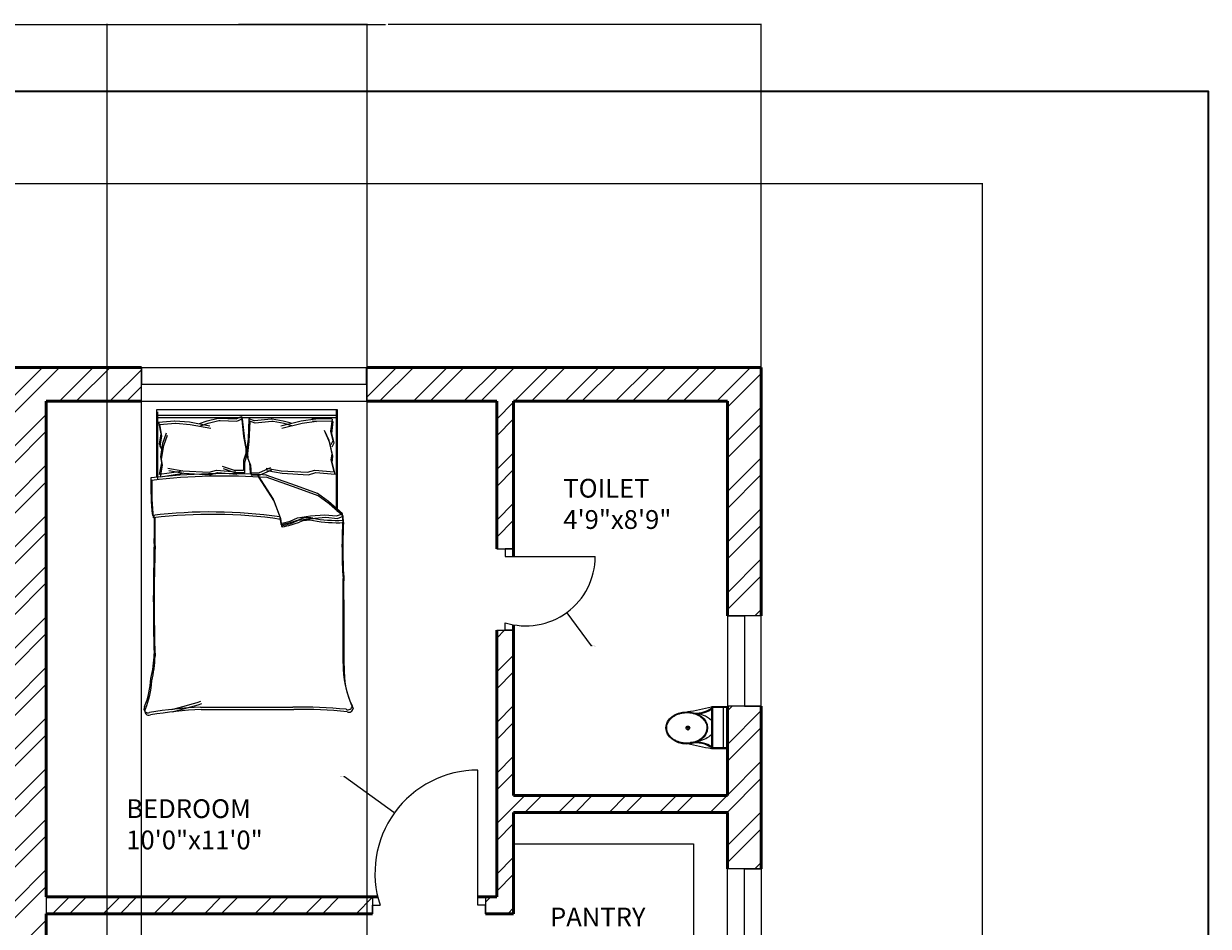
# Model space of a CAD drawing. Units: inches. Extents: x 1896 to 2572, y 1528 to 2474.
# Tile 10 of 10: x 2256 to 2572, y 2234 to 2474. Entities that reach past the tile are written whole.
import ezdxf

# ---------------------------------------------------------------- set-up
doc = ezdxf.new("R2010")
doc.units = ezdxf.units.IN
for name, color, linetype, lineweight in [('A-ANNO-DIMS', 2, 'Continuous', 18), ('A-ANNO-TTLB', 7, 'Continuous', 35), ('A-AREA-IDEN', 7, 'Continuous', 18), ('A-DOOR', 11, 'Continuous', 25), ('A-FLOR-CASE', 7, 'Continuous', 25), ('A-FLOR-FIXT', 8, 'Continuous', 18), ('A-FURN', 8, 'Continuous', 18), ('A-GLAZ', 131, 'Continuous', 20), ('A-WALL', 7, 'Continuous', 50)]:
    doc.layers.add(name, color=color, linetype=linetype, lineweight=lineweight)
doc.layers.add('A-WALL-PATT', color=215, linetype='Continuous', lineweight=13, true_color=0xa953a0)
doc.styles.get("Standard").update_dxf_attribs({"font": 'arial.ttf'})
doc.dimstyles.get("Standard").update_dxf_attribs({"dimtxt": 0.18, "dimasz": 0.18, "dimexe": 0.18, "dimexo": 0.0625, "dimgap": 0.09, "dimtad": 0, "dimtih": 1, "dimtoh": 1, "dimdec": 4, "dimzin": 0, "dimdsep": 46, "dimtxsty": 'Standard', "dimcen": 0.09, "dimadec": 0, "dimazin": 0, "dimtfac": 1, "dimtdec": 4, "dimtofl": 0, "dimtmove": 0, "dimatfit": 3, "dimfxl": 1, "dimtolj": 1, "dimtzin": 0, "dimarcsym": 0})

# ---------------------------------------------------------------- blocks, each defined once
blk = doc.blocks.new('A$C31115884')
for p, q in [((283, 498), (223, 498)), ((258, 466), (258, 523)), ((0, 200), (0, 0)), ((520, 200), (0, 200)), ((10, 190), (10, 10)), ((510, 190), (10, 190)), ((510, 10), (510, 190)), ((520, 0), (520, 200)), ((510, 54), (0, 54)), ((10, 10), (510, 10)), ((0, 0), (520, 0))]:
    blk.add_line(p, q)
blk.add_circle((256, 496), 23.6)
for centre, radius, start, end in [((2778, -205), 2807, 165.4549, 171.7133), ((-295, 403), 365, 324.2091, 9.3499), ((-295, 403), 375, 324.2091, 9.3499), ((806, 403), 365, 170.6501, 215.7909), ((3237, 905), 2807, 188.2867, 194.5451), ((384, 406), 293, 190.2774, 224.1564), ((139, 406), 293, 315.8436, 2.6563), ((806, 403), 375, 179.2036, 215.7909)]:
    blk.add_arc(centre, radius, start, end)
blk.add_ellipse((256, 510), major_axis=(0, -261), ratio=0.772727)
blk.add_open_spline([(256, 259), (263, 259), (270, 260), (288, 262), (299, 265), (320, 273), (330, 278), (350, 291), (360, 299), (378, 316), (386, 326), (402, 347), (409, 358), (421, 383), (427, 395), (436, 422), (440, 436), (445, 465), (447, 480), (448, 509), (448, 524), (445, 553), (443, 568), (436, 596), (432, 610), (422, 636), (416, 649), (402, 672), (395, 683), (379, 703), (370, 712), (351, 728), (341, 735), (321, 746), (310, 751), (289, 757), (278, 759), (256, 761), (245, 761), (223, 757), (212, 754), (191, 746), (181, 741), (161, 728), (151, 720), (133, 703), (125, 693), (110, 672), (103, 660), (90, 636), (85, 623), (76, 596), (72, 582), (67, 553), (66, 538), (64, 509), (65, 494), (68, 465), (70, 450), (77, 422), (81, 408), (91, 382), (97, 370), (111, 346), (118, 335), (135, 316), (144, 307), (162, 291), (172, 284), (193, 273), (203, 269), (225, 262), (236, 260), (250, 259), (253, 259), (256, 259)], degree=3, knots=[0, 0, 0, 0, 0.110105, 0.110105, 0.285049, 0.285049, 0.459994, 0.459994, 0.634938, 0.634938, 0.809882, 0.809882, 0.984827, 0.984827, 1.159771, 1.159771, 1.334715, 1.334715, 1.50966, 1.50966, 1.684604, 1.684604, 1.859549, 1.859549, 2.034493, 2.034493, 2.209437, 2.209437, 2.384382, 2.384382, 2.559326, 2.559326, 2.73427, 2.73427, 2.909215, 2.909215, 3.084159, 3.084159, 3.259103, 3.259103, 3.434048, 3.434048, 3.608992, 3.608992, 3.783936, 3.783936, 3.958881, 3.958881, 4.133825, 4.133825, 4.30877, 4.30877, 4.483714, 4.483714, 4.658658, 4.658658, 4.833603, 4.833603, 5.008547, 5.008547, 5.183491, 5.183491, 5.358436, 5.358436, 5.53338, 5.53338, 5.708324, 5.708324, 5.883269, 5.883269, 6.058213, 6.058213, 6.233158, 6.233158, 6.283185, 6.283185, 6.283185, 6.283185])
blk = doc.blocks.new('BED-DOUBLE')
for p, q in [((3.47, 63.33), (3.47, 81.44)), ((3.47, 63.33), (3.47, 81.44)), ((3.47, 81.44), (51.49, 81.44)), ((3.47, 79.91), (51.27, 79.91)), ((3.47, 79.91), (51.26, 79.91)), ((3.7, 62.69), (3.7, 80.8)), ((3.7, 62.69), (3.7, 80.8)), ((3.7, 79.27), (51.49, 79.27)), ((3.7, 79.27), (51.49, 79.27)), ((16.88, 78.42), (19.77, 79.14)), ((16.88, 78.42), (19.77, 79.14)), ((19.77, 79.14), (20.09, 79.14)), ((19.77, 79.14), (20.09, 79.14)), ((20.09, 79.14), (24.54, 78.99)), ((20.09, 79.14), (24.54, 78.99)), ((24.54, 78.99), (25.98, 79.57)), ((24.54, 78.99), (25.98, 79.57)), ((24.76, 78.36), (26.21, 78.93)), ((24.77, 78.36), (26.21, 78.93)), ((25.98, 79.57), (26.56, 74.22)), ((25.98, 79.57), (26.56, 74.22)), ((26.21, 78.93), (26.79, 73.58)), ((26.21, 78.93), (26.79, 73.58)), ((27.98, 78.95), (27.73, 73.58)), ((27.98, 78.95), (27.73, 73.58)), ((29.46, 78.46), (27.98, 78.95)), ((29.46, 78.46), (27.98, 78.95)), ((34.2, 78.91), (33.88, 78.89)), ((34.2, 78.91), (33.88, 78.89)), ((37.14, 78.37), (34.2, 78.91)), ((37.13, 78.37), (34.2, 78.91)), ((45.71, 78.9), (41.91, 78.37)), ((45.71, 78.9), (41.91, 78.37)), ((50.11, 78.89), (44.71, 78.98)), ((44.71, 78.98), (45.71, 78.9)), ((50.11, 78.89), (44.71, 78.98)), ((44.71, 78.98), (45.71, 78.9)), ((51.26, 81.44), (51.26, 54.83)), ((51.27, 81.44), (51.27, 54.83)), ((51.49, 81.44), (51.49, 80.8)), ((51.49, 80.8), (51.49, 54.19)), ((51.49, 80.8), (51.49, 54.19)), ((3.89, 78.13), (4.47, 74.95)), ((3.89, 78.13), (4.47, 74.95)), ((3.9, 78.11), (8.18, 78.43)), ((3.9, 78.11), (8.18, 78.43)), ((4.12, 77.49), (4.7, 74.31)), ((4.12, 77.49), (4.7, 74.31)), ((4.13, 77.47), (8.41, 77.8)), ((4.13, 77.47), (8.41, 77.8)), ((8.18, 78.43), (8.28, 78.42)), ((8.18, 78.43), (8.28, 78.42)), ((8.28, 78.42), (12.11, 78.13)), ((8.28, 78.42), (12.11, 78.13)), ((8.41, 77.8), (8.51, 77.78)), ((8.41, 77.8), (8.51, 77.78)), ((8.51, 77.78), (12.34, 77.49)), ((8.51, 77.78), (12.34, 77.49)), ((12.11, 78.13), (17.6, 77.12)), ((12.11, 78.13), (17.6, 77.12)), ((12.34, 77.49), (17.83, 76.48)), ((12.34, 77.49), (17.83, 76.48)), ((14.85, 77.69), (16.88, 78.42)), ((14.85, 77.69), (16.88, 78.42)), ((15.08, 77.05), (17.11, 77.78)), ((15.08, 77.05), (17.11, 77.78)), ((17.11, 77.78), (20, 78.5)), ((17.11, 77.78), (20, 78.5)), ((20, 78.5), (20.32, 78.5)), ((20, 78.5), (20.32, 78.5)), ((20.32, 78.5), (24.77, 78.36)), ((20.32, 78.5), (24.76, 78.36)), ((28.21, 78.31), (27.96, 72.94)), ((28.2, 78.31), (27.96, 72.94)), ((29.68, 77.83), (28.2, 78.31)), ((29.68, 77.83), (28.21, 78.31)), ((33.88, 78.89), (29.46, 78.46)), ((33.88, 78.89), (29.46, 78.46)), ((34.11, 78.25), (29.68, 77.83)), ((34.11, 78.25), (29.68, 77.83)), ((34.43, 78.27), (34.11, 78.25)), ((34.43, 78.27), (34.11, 78.25)), ((37.36, 77.73), (34.43, 78.27)), ((37.36, 77.73), (34.43, 78.27)), ((41.91, 78.37), (36.49, 77.02)), ((41.91, 78.37), (36.49, 77.02)), ((42.14, 77.73), (36.72, 76.38)), ((42.14, 77.73), (36.72, 76.38)), ((39.2, 77.77), (37.13, 78.37)), ((39.2, 77.77), (37.14, 78.37)), ((39.43, 77.13), (37.36, 77.73)), ((39.43, 77.13), (37.36, 77.73)), ((45.94, 78.26), (42.14, 77.73)), ((45.94, 78.26), (42.14, 77.73)), ((50.34, 78.25), (44.94, 78.34)), ((44.94, 78.34), (45.94, 78.26)), ((50.34, 78.25), (44.94, 78.34)), ((44.94, 78.34), (45.94, 78.26)), ((49.31, 73.19), (48.13, 75.87)), ((49.31, 73.19), (48.13, 75.87)), ((50.11, 78.89), (49.73, 75.68)), ((50.11, 78.89), (49.73, 75.68)), ((50.34, 78.25), (49.96, 75.04)), ((50.34, 78.25), (49.96, 75.04)), ((4.47, 74.95), (4.04, 72.34)), ((4.47, 74.95), (4.04, 72.34)), ((4.7, 74.31), (4.27, 71.7)), ((4.7, 74.31), (4.27, 71.7)), ((5.05, 72.49), (6.06, 75.24)), ((5.05, 72.49), (6.06, 75.24)), ((5.28, 71.85), (6.29, 74.6)), ((5.28, 71.85), (6.29, 74.6)), ((26.56, 74.22), (27.14, 71.04)), ((26.56, 74.22), (27.14, 71.04)), ((26.79, 73.58), (27.37, 70.4)), ((26.79, 73.58), (27.37, 70.4)), ((27.73, 73.58), (27.35, 70.37)), ((27.73, 73.58), (27.35, 70.37)), ((27.96, 72.94), (27.58, 69.73)), ((27.96, 72.94), (27.58, 69.73)), ((49.54, 72.55), (48.36, 75.23)), ((49.54, 72.55), (48.36, 75.23)), ((50.11, 69.61), (49.31, 73.19)), ((50.11, 69.61), (49.31, 73.19)), ((49.73, 75.68), (50.33, 73.11)), ((49.73, 75.68), (50.33, 73.11)), ((50.33, 73.11), (49.81, 72.06)), ((50.33, 73.11), (49.81, 72.06)), ((49.96, 75.04), (50.56, 72.47)), ((49.96, 75.04), (50.56, 72.47)), ((4.04, 72.34), (4.62, 71.33)), ((4.04, 72.34), (4.62, 71.33)), ((4.27, 71.7), (4.85, 70.69)), ((4.27, 71.7), (4.85, 70.69)), ((4.47, 68.87), (5.05, 72.49)), ((4.47, 68.87), (5.05, 72.49)), ((4.7, 68.23), (5.28, 71.85)), ((4.7, 68.23), (5.28, 71.85)), ((27.14, 69.74), (26.56, 67.86)), ((27.14, 69.74), (26.56, 67.86)), ((27.14, 71.04), (27.14, 69.74)), ((27.14, 71.04), (27.14, 69.74)), ((27.35, 70.37), (27.44, 69.07)), ((27.35, 70.37), (27.44, 69.07)), ((27.37, 70.4), (27.37, 69.1)), ((27.37, 70.4), (27.37, 69.1)), ((27.58, 69.73), (27.66, 68.43)), ((27.58, 69.73), (27.66, 68.43)), ((50.34, 68.98), (49.54, 72.55)), ((50.34, 68.98), (49.54, 72.55)), ((49.92, 68.01), (50.11, 69.61)), ((49.92, 68.01), (50.11, 69.61)), ((50.56, 72.47), (50.04, 71.42)), ((50.56, 72.47), (50.04, 71.42)), ((4.18, 64.1), (4.76, 67.28)), ((4.18, 64.1), (4.76, 67.28)), ((4.41, 63.46), (4.99, 66.64)), ((4.41, 63.46), (4.99, 66.64)), ((4.76, 67.28), (4.47, 68.87)), ((4.76, 67.28), (4.47, 68.87)), ((4.99, 66.64), (4.7, 68.23)), ((4.99, 66.64), (4.7, 68.23)), ((26.56, 67.86), (26.56, 65.18)), ((26.56, 67.86), (26.56, 65.18)), ((27.37, 69.1), (26.79, 67.22)), ((27.37, 69.1), (26.79, 67.22)), ((26.79, 67.22), (26.79, 64.54)), ((26.79, 67.22), (26.79, 64.54)), ((27.44, 69.07), (28.13, 67.23)), ((27.44, 69.07), (28.13, 67.23)), ((27.66, 68.43), (28.36, 66.59)), ((27.66, 68.43), (28.36, 66.59)), ((28.13, 67.23), (28.3, 64.55)), ((28.13, 67.23), (28.3, 64.55)), ((28.36, 66.59), (28.53, 63.91)), ((28.36, 66.59), (28.53, 63.91)), ((50.7, 64.87), (49.92, 68.01)), ((50.7, 64.87), (49.92, 68.01)), ((50.15, 67.37), (50.34, 68.98)), ((50.15, 67.37), (50.34, 68.98)), ((50.93, 64.23), (50.15, 67.37)), ((50.93, 64.23), (50.15, 67.37)), ((9.28, 64.83), (4.18, 64.1)), ((9.28, 64.83), (4.18, 64.1)), ((9.51, 64.19), (4.41, 63.46)), ((9.51, 64.19), (4.41, 63.46)), ((6.38, 65.81), (10.41, 65.15)), ((6.38, 65.81), (10.41, 65.15)), ((6.61, 65.18), (10.64, 64.51)), ((6.61, 65.18), (10.64, 64.51)), ((10.41, 65.15), (9.28, 64.83)), ((10.41, 65.15), (9.28, 64.83)), ((10.64, 64.51), (9.51, 64.19)), ((10.64, 64.51), (9.51, 64.19)), ((10.41, 65.15), (17.42, 64.72)), ((10.41, 65.15), (17.42, 64.72)), ((10.64, 64.51), (17.65, 64.08)), ((10.64, 64.51), (17.65, 64.08)), ((17.42, 64.72), (19.38, 65.27)), ((17.42, 64.72), (19.38, 65.27)), ((17.65, 64.08), (19.61, 64.63)), ((17.65, 64.08), (19.61, 64.63)), ((19.38, 65.27), (24.52, 64.87)), ((19.38, 65.27), (24.52, 64.87)), ((19.61, 64.63), (24.74, 64.23)), ((19.61, 64.63), (24.74, 64.23)), ((24.1, 65.18), (20.96, 66.27)), ((24.1, 65.18), (20.96, 66.27)), ((24.33, 64.54), (21.19, 65.63)), ((24.33, 64.54), (21.19, 65.63)), ((26.56, 65.18), (24.1, 65.18)), ((26.56, 65.18), (24.1, 65.18)), ((26.79, 64.54), (24.33, 64.54)), ((26.79, 64.54), (24.33, 64.54)), ((28.3, 64.55), (30.75, 64.7)), ((28.3, 64.55), (30.75, 64.7)), ((28.53, 63.91), (30.98, 64.06)), ((28.53, 63.91), (30.98, 64.06)), ((30.26, 64.06), (34.45, 57.57)), ((30.26, 64.06), (34.45, 57.57)), ((30.49, 63.42), (34.68, 56.93)), ((30.49, 63.42), (34.68, 56.93)), ((30.75, 64.7), (33.82, 65.99)), ((30.75, 64.7), (33.82, 65.99)), ((30.98, 64.06), (34.05, 65.35)), ((30.98, 64.06), (34.05, 65.35)), ((40.64, 61.13), (32.31, 64.06)), ((40.64, 61.13), (32.31, 64.06)), ((40.87, 60.49), (32.53, 63.42)), ((40.87, 60.49), (32.53, 63.42)), ((32.56, 65.81), (36.6, 65.15)), ((32.56, 65.81), (36.6, 65.15)), ((32.79, 65.18), (36.82, 64.51)), ((32.79, 65.18), (36.82, 64.51)), ((36.6, 65.15), (43.61, 64.72)), ((36.6, 65.15), (43.61, 64.72)), ((36.82, 64.51), (43.83, 64.08)), ((36.82, 64.51), (43.83, 64.08)), ((43.61, 64.72), (45.57, 65.27)), ((43.61, 64.72), (45.57, 65.27)), ((43.83, 64.08), (45.79, 64.63)), ((43.83, 64.08), (45.79, 64.63)), ((45.57, 65.27), (50.7, 64.87)), ((45.57, 65.27), (50.7, 64.87)), ((45.79, 64.63), (50.93, 64.23)), ((45.79, 64.63), (50.93, 64.23)), ((46.22, 59.11), (40.64, 61.13)), ((46.22, 59.11), (40.64, 61.13)), ((46.45, 58.48), (40.87, 60.49)), ((46.45, 58.48), (40.87, 60.49)), ((34.45, 57.57), (36.15, 53.08)), ((34.45, 57.57), (36.15, 53.08)), ((34.68, 56.93), (36.38, 52.44)), ((34.68, 56.93), (36.38, 52.44)), ((49.16, 56.95), (46.22, 59.11)), ((49.16, 56.95), (46.22, 59.11)), ((49.39, 56.31), (46.45, 58.48)), ((49.39, 56.31), (46.45, 58.48)), ((52.87, 53.7), (49.16, 56.95)), ((52.87, 53.7), (49.16, 56.95)), ((53.1, 53.06), (49.39, 56.31)), ((53.1, 53.06), (49.39, 56.31)), ((51.33, 53.08), (52.87, 53.7)), ((51.33, 53.08), (52.87, 53.7)), ((52.95, 51.95), (52.87, 53.7, 3.87)), ((52.95, 51.95), (52.87, 53.7, 3.87)), ((36.15, 53.08), (36.46, 51.07)), ((36.15, 53.08), (36.46, 51.07)), ((36.38, 52.44), (36.69, 50.43)), ((36.38, 52.44), (36.69, 50.43)), ((36.46, 51.07), (38.94, 51.69)), ((36.46, 51.07), (38.94, 51.69)), ((36.69, 50.43), (39.17, 51.05)), ((36.69, 50.43), (39.17, 51.05)), ((38.94, 51.69), (40.95, 52.61)), ((38.94, 51.69), (40.95, 52.61)), ((39.17, 51.05), (41.18, 51.97)), ((39.17, 51.05), (41.18, 51.97)), ((40.95, 52.61), (44.36, 53.08)), ((40.95, 52.61), (44.36, 53.08)), ((41.18, 51.97), (44.59, 52.44)), ((41.18, 51.97), (44.59, 52.44)), ((44.36, 53.08), (48.23, 53.39)), ((44.36, 53.08), (48.23, 53.39)), ((44.59, 52.44), (48.46, 52.75)), ((44.59, 52.44), (48.46, 52.75)), ((48.23, 53.39), (51.33, 53.08)), ((48.23, 53.39), (51.33, 53.08)), ((48.46, 52.75), (51.56, 52.44)), ((48.46, 52.75), (51.56, 52.44)), ((51.56, 52.44), (53.1, 53.06)), ((51.56, 52.44), (53.1, 53.06)), ((53.18, 51.31), (53.1, 53.06, 3.87)), ((53.17, 51.31), (53.1, 53.06, 3.87)), ((15.06, 2.2), (39.68, 2.2)), ((15.06, 2.2), (39.68, 2.2)), ((15.29, 1.56), (39.91, 1.56)), ((15.29, 1.56), (39.91, 1.56))]:
    blk.add_line(p, q)
for centre, radius, start, end in [((85.16, 61.35), 83.31, 178.7218, 185.604), ((85.16, 61.35), 83.31, 178.7218, 185.604), ((21.36, -100.61), 164.97, 86.0865, 96.7821), ((21.36, -100.61), 164.97, 86.0865, 96.7821), ((21.59, -101.25), 164.97, 86.0865, 96.7821), ((21.59, -101.25), 164.97, 86.0865, 96.7821), ((85.39, 60.71), 83.31, 178.7218, 185.604), ((85.39, 60.71), 83.31, 178.7218, 185.604), ((17.76, -74.87), 129.02, 81.7845, 96.9006), ((17.76, -74.87), 129.02, 81.7845, 96.9006), ((17.98, -75.51), 129.02, 81.7845, 96.9006), ((17.98, -75.51), 129.02, 81.7845, 96.9006), ((-167.31, 50.27), 170.11, 358.4762, 1.0082), ((-167.31, 50.27), 170.11, 358.4762, 1.0082), ((-167.08, 49.63), 170.11, 358.4762, 1.0082), ((-167.08, 49.63), 170.11, 358.4762, 1.0082), ((36.64, 51), 0.185, 160.2464, 271.1377), ((36.64, 51), 0.185, 160.2464, 271.1377), ((31.15, 79.96), 29.65, 280.6617, 289.8806), ((31.15, 79.96), 29.65, 280.6617, 289.8806), ((31.38, 79.32), 29.65, 280.6617, 289.8806), ((31.38, 79.32), 29.65, 280.6617, 289.8806), ((43.74, 46.38), 6.22, 78.6608, 113.7384), ((43.74, 46.38), 6.22, 78.6608, 113.7384), ((43.97, 45.74), 6.22, 78.6608, 113.7384), ((43.97, 45.74), 6.22, 78.6608, 113.7384), ((51.33, 88.1), 36.18, 259.8763, 272.5657), ((51.33, 88.1), 36.18, 259.8763, 272.5657), ((51.56, 87.46), 36.18, 259.8763, 272.5657), ((51.56, 87.46), 36.18, 259.8763, 272.5657), ((182.27, 45.13), 129.5, 176.9791, 183.8365), ((182.27, 45.13), 129.5, 176.9791, 183.8365), ((182.49, 44.49), 129.5, 176.9791, 183.8365), ((182.49, 44.49), 129.5, 176.9791, 183.8365), ((36.86, 50.36), 0.185, 160.2464, 271.1377), ((36.86, 50.36), 0.185, 160.2464, 271.1377), ((484.82, 30.83), 482.31, 178.2277, 181.7185), ((484.82, 30.83), 482.31, 178.2277, 181.7185), ((485.05, 30.19), 482.31, 178.2277, 181.7185), ((485.05, 30.19), 482.31, 178.2277, 181.7185), ((-4508.74, 13.62), 4561.86, 0.00217, 0.28689), ((-4508.74, 13.62), 4561.86, 0.00217, 0.28689), ((-4508.52, 12.98), 4561.86, 0.00217, 0.28689), ((-4508.52, 12.98), 4561.86, 0.00217, 0.28689), ((-26.9, 16.93), 29.63, 346.0648, 358.9113), ((-26.9, 16.93), 29.63, 346.0648, 358.9113), ((-26.67, 16.29), 29.63, 346.0648, 358.9113), ((-26.67, 16.29), 29.63, 346.0648, 358.9113), ((76.16, 12.78), 23.07, 177.4714, 206.4681), ((76.16, 12.78), 23.07, 177.4714, 206.4681), ((76.39, 12.14), 23.07, 177.4714, 206.4681), ((76.39, 12.14), 23.07, 177.4714, 206.4681), ((-21.66, 11.17), 23.56, 337.9751, 356.652), ((-21.66, 11.17), 23.56, 337.9751, 356.652), ((-21.43, 10.53), 23.56, 337.9751, 356.652), ((-21.43, 10.53), 23.56, 337.9751, 356.652), ((-17.22, 105.16), 106.46, 283.3832, 287.7053), ((-17.22, 105.16), 106.46, 283.3832, 287.7053), ((1.09, 1.73), 1.09, 146.1736, 293.4781), ((1.09, 1.73), 1.09, 146.1736, 293.4781), ((1.32, 1.09), 1.09, 146.1736, 293.4781), ((1.32, 1.09), 1.09, 146.1736, 293.4781), ((21.43, -119.39), 121.76, 92.9958, 99.4091), ((21.43, -119.39), 121.76, 92.9958, 99.4091), ((21.65, -120.03), 121.76, 92.9958, 99.4091), ((21.65, -120.03), 121.76, 92.9958, 99.4091), ((-16.99, 104.52), 106.46, 283.3832, 287.7053), ((-16.99, 104.52), 106.46, 283.3832, 287.7053), ((41.15, -130.83), 133.04, 84.4998, 90.6351), ((41.15, -130.83), 133.04, 84.4998, 90.6351), ((41.38, -131.47), 133.04, 84.4998, 90.6351), ((41.38, -131.47), 133.04, 84.4998, 90.6351), ((54.41, 2.57), 1.1, 242.6588, 356.02), ((54.41, 2.57), 1.1, 242.6588, 356.02), ((54.64, 1.93), 1.1, 242.6588, 356.02), ((54.64, 1.93), 1.1, 242.6588, 356.02)]:
    blk.add_arc(centre, radius, start, end)
blk = doc.blocks.new('WIN-24IN')
for p, q in [((4.5, 24), (0, 24)), ((0, 24), (9, 24)), ((0, 24), (0, 0)), ((4.5, 0), (4.5, 24)), ((9, 0), (9, 24)), ((0, 0), (9, 0)), ((9, 0), (4.5, 0))]:
    blk.add_line(p, q)
blk = doc.blocks.new('WIN-36IN')
for p, q in [((0, 36), (9, 36)), ((0, 0), (0, 36)), ((9, 36), (4.5, 36)), ((4.5, 36), (4.5, 0)), ((9, 36), (9, 0)), ((4.5, 0), (0, 0)), ((0, 0), (9, 0))]:
    blk.add_line(p, q)
blk = doc.blocks.new('*D20')
at = {"layer": 'A-ANNO-DIMS', "color": 0, "lineweight": -2, "transparency": 16777216}
for p, q in [((2180.68, 2431.4), (2511.65, 2431.4)), ((2511.47, 2431.22), (2511.47, 2049.83)), ((2511.47, 1668.08), (2511.47, 2049.47)), ((2452.68, 1667.9), (2511.65, 1667.9))]:
    blk.add_line(p, q, dxfattribs=at)
at = {"layer": 'A-ANNO-DIMS', "color": 0, "transparency": 16777216}
for points in [[(2511.44, 2431.22), (2511.5, 2431.22), (2511.47, 2431.4)], [(2511.44, 1668.08), (2511.5, 1668.08), (2511.47, 1667.9)]]:
    blk.add_solid(points, dxfattribs=at)
at = {"layer": 'Defpoints', "color": 0, "transparency": 16777216}
for p in [(2180.62, 2431.4), (2511.47, 2431.4), (2452.62, 1667.9)]:
    blk.add_point(p, dxfattribs=at)
at = {"layer": 'A-ANNO-DIMS', "color": 0, "transparency": 16777216, "insert": (2511.47, 2049.65), "char_height": 0.18, "attachment_point": 5}
blk.add_mtext('\\A1;763.5', dxfattribs=at)
blk = doc.blocks.new('*D24')
at = {"layer": 'A-ANNO-DIMS', "color": 0, "lineweight": -2, "transparency": 16777216}
for p, q in [((2253.12, 2373.46), (2253.12, 2473.93)), ((2253.3, 2473.75), (2352.49, 2473.75)), ((2452.44, 2473.75), (2353.26, 2473.75)), ((2452.62, 2382.46), (2452.62, 2473.93))]:
    blk.add_line(p, q, dxfattribs=at)
at = {"layer": 'A-ANNO-DIMS', "color": 0, "transparency": 16777216}
for points in [[(2253.3, 2473.78), (2253.3, 2473.72), (2253.12, 2473.75)], [(2452.44, 2473.78), (2452.44, 2473.72), (2452.62, 2473.75)]]:
    blk.add_solid(points, dxfattribs=at)
at = {"layer": 'Defpoints', "color": 0, "transparency": 16777216}
for p in [(2452.62, 2473.75), (2452.62, 2382.4), (2253.12, 2373.4)]:
    blk.add_point(p, dxfattribs=at)
at = {"layer": 'A-ANNO-DIMS', "color": 0, "transparency": 16777216, "insert": (2352.87, 2473.75), "char_height": 0.18, "attachment_point": 5}
blk.add_mtext('\\A1;199.5', dxfattribs=at)
blk = doc.blocks.new('*D29')
at = {"layer": 'A-ANNO-DIMS', "color": 0, "lineweight": -2, "transparency": 16777216}
for p, q in [((2278.35, 2039.96), (2278.35, 2473.93)), ((2278.53, 2473.75), (2312.59, 2473.75)), ((2347.44, 2473.75), (2313.38, 2473.75)), ((2347.62, 2039.96), (2347.62, 2473.93))]:
    blk.add_line(p, q, dxfattribs=at)
at = {"layer": 'A-ANNO-DIMS', "color": 0, "transparency": 16777216}
for points in [[(2278.53, 2473.78), (2278.53, 2473.72), (2278.35, 2473.75)], [(2347.44, 2473.78), (2347.44, 2473.72), (2347.62, 2473.75)]]:
    blk.add_solid(points, dxfattribs=at)
at = {"layer": 'Defpoints', "color": 0, "transparency": 16777216}
for p in [(2347.62, 2473.75), (2278.35, 2039.9), (2347.62, 2039.9)]:
    blk.add_point(p, dxfattribs=at)
at = {"layer": 'A-ANNO-DIMS', "color": 0, "transparency": 16777216, "insert": (2312.99, 2473.75), "char_height": 0.18, "attachment_point": 5}
blk.add_mtext('\\A1;69.27', dxfattribs=at)
blk = doc.blocks.new('*D35')
at = {"layer": 'A-ANNO-DIMS', "color": 0, "lineweight": -2, "transparency": 16777216}
for p, q in [((2262.12, 2373.34), (2262.12, 1549.1)), ((2287.46, 2373.34), (2287.46, 1549.1)), ((2262.3, 1549.28), (2274.4, 1549.28)), ((2287.28, 1549.28), (2275.19, 1549.28))]:
    blk.add_line(p, q, dxfattribs=at)
at = {"layer": 'A-ANNO-DIMS', "color": 0, "transparency": 16777216}
for points in [[(2262.3, 1549.31), (2262.3, 1549.25), (2262.12, 1549.28)], [(2287.28, 1549.31), (2287.28, 1549.25), (2287.46, 1549.28)]]:
    blk.add_solid(points, dxfattribs=at)
at = {"layer": 'Defpoints', "color": 0, "transparency": 16777216}
for p in [(2262.12, 2373.4), (2287.46, 2373.4), (2287.46, 1549.28)]:
    blk.add_point(p, dxfattribs=at)
at = {"layer": 'A-ANNO-DIMS', "color": 0, "transparency": 16777216, "insert": (2274.79, 1549.28), "char_height": 0.18, "attachment_point": 5}
blk.add_mtext('\\A1;25.34', dxfattribs=at)
blk = doc.blocks.new('*D42')
at = {"layer": 'A-ANNO-DIMS', "color": 0, "lineweight": -2, "transparency": 16777216}
for p, q in [((2341.4, 2273.45), (2341.58, 2273.45)), ((2341.58, 2273.45), (2354.77, 2263.91)), ((2377.04, 2247.72), (2377.22, 2247.72)), ((2377.13, 2247.63), (2377.13, 2247.81))]:
    blk.add_line(p, q, dxfattribs=at)
at = {"layer": 'A-ANNO-DIMS', "color": 0, "transparency": 16777216}
blk.add_solid([(2354.78, 2263.93), (2354.75, 2263.88), (2354.91, 2263.8)], dxfattribs=at)
at = {"layer": 'Defpoints', "color": 0, "transparency": 16777216}
for p in [(2354.91, 2263.8), (2377.13, 2247.72)]:
    blk.add_point(p, dxfattribs=at)
at = {"layer": 'A-ANNO-DIMS', "color": 0, "transparency": 16777216, "insert": (2340.92, 2273.45), "char_height": 0.18, "attachment_point": 5}
blk.add_mtext('\\A1;R27.43', dxfattribs=at)
blk = doc.blocks.new('*D50')
at = {"layer": 'A-ANNO-DIMS', "color": 0, "lineweight": -2, "transparency": 16777216}
for p, q in [((2389.81, 2332.03), (2389.99, 2332.03)), ((2389.9, 2331.94), (2389.9, 2332.12)), ((2407.4, 2308.21), (2400.94, 2317)), ((2407.58, 2308.21), (2407.4, 2308.21))]:
    blk.add_line(p, q, dxfattribs=at)
at = {"layer": 'A-ANNO-DIMS', "color": 0, "transparency": 16777216}
blk.add_solid([(2400.97, 2317.02), (2400.92, 2316.98), (2400.83, 2317.14)], dxfattribs=at)
at = {"layer": 'Defpoints', "color": 0, "transparency": 16777216}
for p in [(2389.9, 2332.03), (2400.83, 2317.14)]:
    blk.add_point(p, dxfattribs=at)
at = {"layer": 'A-ANNO-DIMS', "color": 0, "transparency": 16777216, "insert": (2408.13, 2308.21), "char_height": 0.18, "attachment_point": 5}
blk.add_mtext('\\A1;R18.475', dxfattribs=at)

msp = doc.modelspace()

# ---------------------------------------------------------------- hatches: boundary and pattern name
at = {"layer": 'A-WALL-PATT'}
h = msp.add_hatch(dxfattribs=at)
h.set_pattern_fill('ANSI32', color=256)
h.paths.add_polyline_path([(2071.6224, 2382.3979), (2071.6224, 2422.3979), (2110.6224, 2422.3979), (2110.6224, 2382.3979), (2110.6224, 2357.5961), (2119.6224, 2357.5961), (2119.6224, 2422.3979), (2171.6224, 2422.3979), (2171.6224, 2373.3979), (2193.5093, 2373.3979), (2193.5093, 2377.8979), (2193.5093, 2382.3979), (2180.6224, 2382.3979), (2180.6224, 2431.3979), (2171.6224, 2431.3979), (2119.6224, 2431.3979), (2110.6224, 2431.3979), (2062.6224, 2431.3979), (2062.6224, 2422.3979), (2062.6224, 2382.3979), (1978.6224, 2382.3979), (1978.6224, 2313.0337), (1987.6224, 2313.0337), (1987.6224, 2373.3979), (2062.6224, 2373.3979), (2067.1224, 2373.3979), (2067.1224, 2353.7982), (2071.6224, 2353.8883)])
h.paths.add_polyline_path([(2287.4624, 2382.3979), (2229.5093, 2382.3979), (2229.5093, 2373.3979), (2253.1224, 2373.3979), (2253.1224, 2175.8979), (2247.1039, 2175.8979), (2247.1039, 2166.8979), (2253.1224, 2166.8979), (2253.1224, 2150.8283), (2262.1224, 2150.8283), (2262.1224, 2166.8979), (2262.1224, 2236.8979), (2349.0731, 2236.8979), (2349.0731, 2239.1479), (2349.0731, 2241.3979), (2262.1224, 2241.3979), (2262.1224, 2373.3979), (2287.4624, 2373.3979)])
h.paths.add_polyline_path([(2452.6224, 2382.3979), (2347.4624, 2382.3979), (2347.4624, 2373.3979), (2382.1224, 2373.3979), (2382.1224, 2334.0335), (2386.6224, 2334.0335), (2386.6224, 2373.3979), (2443.6224, 2373.3979), (2443.6224, 2316.2056), (2452.6224, 2316.2056)])
h.paths.add_polyline_path([(2452.6224, 2292.2056), (2448.1224, 2292.2056), (2443.6224, 2292.2056), (2443.6224, 2292.0047), (2443.6224, 2280.9372), (2443.6224, 2268.3979), (2386.6224, 2268.3979), (2386.6224, 2312.4044), (2384.3724, 2312.4044), (2382.1224, 2312.4044), (2382.1224, 2241.3979), (2379.1336, 2241.3979), (2379.1336, 2236.8979), (2386.6224, 2236.8979), (2386.6224, 2263.8979), (2443.6224, 2263.8979), (2443.6224, 2248.8449), (2452.6224, 2248.8449)])
h.paths.add_polyline_path([(2364.1285, 2116.8979), (2262.1224, 2116.8979), (2262.1224, 2120.5401), (2257.6224, 2120.5401), (2253.1224, 2120.5401), (2253.1224, 2107.8979), (2262.1224, 2107.8979), (2269.354, 2107.8979), (2269.354, 2094.0702), (2278.354, 2094.0702), (2278.354, 2107.8979), (2347.6224, 2107.8979), (2347.6224, 2039.8979), (2278.354, 2039.8979), (2278.354, 2054.7605), (2269.354, 2054.7605), (2269.354, 2030.8979), (2278.354, 2030.8979), (2443.6224, 2030.8979), (2443.6224, 2015.198), (2452.6224, 2015.198), (2452.6224, 2030.8979), (2464.6224, 2030.8979), (2469.1224, 2030.8979), (2469.1224, 2117.0352), (2452.6767, 2116.9466), (2452.6285, 2125.8979), (2452.6224, 2125.8979), (2452.6224, 2212.8449), (2443.6224, 2212.8449), (2443.6224, 2116.8979), (2385.832, 2116.8979), (2385.832, 2112.3979), (2385.832, 2107.8979), (2464.6224, 2107.8979), (2464.6224, 2039.8979), (2443.6224, 2039.8979), (2356.6224, 2039.8979), (2356.6224, 2107.8979), (2364.1285, 2107.8979)])
h.paths.add_polyline_path([(2452.6224, 1967.198), (2443.6224, 1967.198), (2443.6224, 1955.8979), (2259.1224, 1955.8979), (2254.6224, 1955.8979), (2254.6224, 1941.6358), (2263.6224, 1941.6358), (2263.6224, 1946.8979), (2379.1224, 1946.8979), (2379.1224, 1913.0204), (2383.6224, 1913.0204), (2383.6224, 1946.8979), (2443.6224, 1946.8979), (2443.6224, 1930.729), (2452.6224, 1930.729)])
h.paths.add_polyline_path([(2469.1224, 1871.8979), (2464.6224, 1871.8979), (2452.6224, 1871.8979), (2452.6224, 1894.729), (2443.6224, 1894.729), (2443.6224, 1871.8979), (2388.1304, 1871.8979), (2388.1304, 1867.3979), (2443.6224, 1867.3979), (2464.6224, 1867.3979), (2464.6224, 1817.8979), (2443.6224, 1817.8979), (2388.1304, 1817.8979), (2388.1304, 1815.6479), (2388.1304, 1813.3979), (2391.1224, 1813.3979), (2391.1224, 1747.8899), (2395.6224, 1747.8899), (2395.6224, 1813.3979), (2443.6224, 1813.3979), (2443.6224, 1781.4434), (2452.6224, 1781.4434), (2452.6224, 1813.3979), (2464.6224, 1813.3979), (2469.1224, 1813.3979)])
h.paths.add_polyline_path([(2263.6224, 1910.9737), (2259.1224, 1910.9737), (2254.6224, 1910.9737), (2254.6224, 1889.8979), (2251.2778, 1889.8979), (2251.2778, 1880.8979), (2254.6224, 1880.8979), (2254.6224, 1817.8979), (2254.6224, 1754.8979), (2254.6224, 1693.3979), (2254.6224, 1684.3979), (2254.6224, 1672.3979), (2200.6224, 1672.3979), (2200.6224, 1684.3979), (2200.6224, 1693.3979), (2200.6224, 1754.8979), (2196.1224, 1754.8979), (2196.1224, 1693.3979), (2150.0488, 1693.3979), (2150.0488, 1684.3979), (2196.1224, 1684.3979), (2196.1224, 1672.3979), (2196.1224, 1667.8979), (2254.6224, 1667.8979), (2259.1224, 1667.8979), (2259.1224, 1693.3979), (2259.1224, 1813.3979), (2353.6224, 1813.3979), (2353.6224, 1815.6479), (2353.6224, 1817.8979), (2263.6224, 1817.8979)])
h.paths.add_polyline_path([(2391.1224, 1693.3979), (2345.6981, 1693.3979), (2345.6981, 1684.3979), (2391.1224, 1684.3979)])
h.paths.add_polyline_path([(2285.6981, 1693.3979), (2259.1224, 1693.3979), (2259.1224, 1684.3979), (2285.6981, 1684.3979), (2285.6981, 1688.8979)], flags=17)
h.paths.add_polyline_path([(2452.6224, 1757.4434), (2448.1224, 1757.4434), (2443.6224, 1757.4434), (2443.6224, 1726.3979), (2395.6224, 1726.3979), (2395.6224, 1728.6572), (2393.3724, 1728.6572), (2391.1224, 1728.6572), (2391.1224, 1717.6723), (2395.6224, 1717.6723), (2395.6224, 1721.8979), (2443.6224, 1721.8979), (2443.6224, 1714.8), (2452.6224, 1714.8)])
h.paths.add_polyline_path([(2452.6224, 1684.3979), (2452.6224, 1690.8), (2443.6224, 1690.8), (2443.6224, 1679.8979), (2443.6224, 1672.3979), (2395.6224, 1672.3979), (2395.6224, 1695.6708), (2391.1224, 1695.5986), (2391.1224, 1672.3979), (2391.1224, 1667.8979), (2452.6224, 1667.8979)])
h.paths.add_polyline_path([(1987.6224, 1880.8979), (2068.6224, 1880.8979), (2125.6224, 1880.8979), (2125.6224, 1788.8466), (2130.1224, 1788.8466), (2130.1224, 1880.8979), (2216.1958, 1880.8979), (2216.1958, 1885.3979), (2216.1958, 1889.8979), (2208.1224, 1889.8979), (2208.1224, 1996.3717), (2203.6224, 1996.3717), (2199.1224, 1996.3717), (2199.1224, 1889.8979), (2073.1224, 1889.8979), (2073.1224, 1917.1874), (2068.6224, 1917.1874), (2068.6224, 1889.8979), (1987.6224, 1889.8979), (1987.6224, 1912.4976), (1978.6224, 1912.4976), (1978.6224, 1805.5193), (1987.6224, 1805.5193)])
h.paths.add_polyline_path([(2019.9303, 1754.8979), (1987.6224, 1754.8979), (1966.6224, 1754.8979), (1966.6224, 1801.0193), (1987.6224, 1801.0193), (1987.6224, 1805.5193), (1962.1224, 1805.5193), (1962.1224, 1750.3979), (1966.6224, 1750.3979), (1978.6224, 1750.3979), (1987.6224, 1750.3979), (2019.9303, 1750.3979)])
h.paths.add_polyline_path([(2135.5566, 1754.8979), (2130.1224, 1754.8979), (2130.1224, 1758.052), (2127.8724, 1758.052), (2125.6224, 1758.052), (2125.6224, 1754.8979), (2068.6224, 1754.8979), (2043.2292, 1754.8979), (2043.2292, 1750.3979), (2068.6224, 1750.3979), (2098.6224, 1750.3979), (2098.6224, 1693.3979), (2068.6224, 1693.3979), (1987.6224, 1693.3979), (1987.6224, 1707.3003), (1983.1224, 1707.3003), (1978.6224, 1707.3003), (1978.6224, 1684.3979), (2068.6224, 1684.3979), (2126.0488, 1684.3979), (2126.0488, 1688.8979), (2126.0488, 1693.3979), (2103.1224, 1693.3979), (2103.1224, 1750.3979), (2130.1224, 1750.3979), (2135.5566, 1750.3979)])
h.paths.add_polyline_path([(1987.6224, 1750.3979), (1978.6224, 1750.3979), (1978.6224, 1731.3003), (1987.6224, 1731.3003)], flags=0)
h.paths.add_polyline_path([(1987.6224, 1973.8979), (2068.6224, 1973.8979), (2073.1224, 1973.8979), (2073.1224, 1978.3979), (1971.1224, 1978.3979), (1971.1224, 2030.3979), (1978.6224, 2030.3979), (1987.6224, 2030.3979), (2104.9199, 2030.3979), (2104.9199, 2032.6479), (2104.9199, 2034.8979), (1987.6224, 2034.8979), (1971.1224, 2034.8979), (1971.1224, 2085.8979), (2003.6464, 2085.8979), (2003.6464, 2090.3979), (1987.6224, 2090.3979), (1987.6224, 2166.8979), (2115.1224, 2166.8979), (2137.6224, 2166.8979), (2137.6224, 2114.4229), (2142.1224, 2114.4229), (2142.1224, 2124.8979), (2153.5306, 2124.8979), (2153.5306, 2127.1479), (2153.5306, 2129.3979), (2142.1224, 2129.3979), (2142.1224, 2166.8979), (2199.1224, 2166.8979), (2199.1224, 2129.3979), (2177.5306, 2129.3979), (2177.5306, 2124.8979), (2199.1224, 2124.8979), (2199.1224, 2034.8979), (2142.1224, 2034.8979), (2142.1224, 2091.6671), (2139.8724, 2091.6671), (2137.6224, 2091.6671), (2137.6224, 2034.8979), (2133.8326, 2034.8979), (2133.8326, 2030.3979), (2137.6224, 2030.3979), (2142.1224, 2030.3979), (2199.1224, 2030.3979), (2199.1224, 2024.2654), (2208.1224, 2024.2654), (2208.1224, 2030.3979), (2208.1224, 2166.8979), (2214.5775, 2166.8979), (2214.5775, 2171.3979), (2214.5775, 2175.8979), (2115.1224, 2175.8979), (2115.1224, 2329.9154), (2112.4137, 2329.9154), (2110.6224, 2329.9154), (2110.6224, 2175.8979), (2082.1224, 2175.8979), (2082.1224, 2202.6443), (2079.8724, 2202.6443), (2077.6224, 2202.6443), (2077.6224, 2175.8979), (1987.6224, 2175.8979), (1987.6224, 2191.3531), (1983.1224, 2191.3531), (1978.6224, 2191.3531), (1978.6224, 2090.3979), (1966.6224, 2090.3979), (1966.6224, 2085.8979), (1966.6224, 2030.3979), (1966.6224, 1973.8979), (1978.6224, 1973.8979), (1978.6224, 1948.4976), (1983.1224, 1948.4976), (1987.6224, 1948.4976)])
h.paths.add_polyline_path([(1987.6224, 2253.0337), (1983.1224, 2253.0337), (1978.6224, 2253.0337), (1978.6224, 2215.3531), (1987.6224, 2215.3531), (1987.6224, 2224.8979), (2077.6224, 2224.8979), (2077.6224, 2221.9854), (2082.1224, 2221.9854), (2082.1224, 2229.3979), (1987.6224, 2229.3979)], flags=17)
h.paths.add_polyline_path([(2220.5047, 1978.7278), (2253.7278, 1978.7278), (2253.7278, 1997.3851), (2220.5047, 1997.3851)], flags=9)
h.paths.add_polyline_path([(2303.6746, 2064.9806), (2320.5334, 2064.9806), (2320.5334, 2075.2842), (2303.6746, 2075.2842)], flags=25)

# ---------------------------------------------------------------- linework, layer by layer
at = {"layer": 'A-ANNO-TTLB'}
msp.add_lwpolyline([(1895.84, 2455.9668), (2571.702, 2455.9668), (2571.702, 1527.8833), (1895.84, 1527.8833)], close=True, dxfattribs=at)
at = {"layer": 'A-DOOR'}
for p, q in [((2382.1224, 2334.0335), (2386.6224, 2334.0335)), ((2386.6224, 2334.0335), (2384.3724, 2334.0335)), ((2384.3724, 2334.0335), (2384.3724, 2332.0335)), ((2384.3724, 2332.0335), (2408.3724, 2332.0335)), ((2384.3724, 2312.4044), (2384.3724, 2314.4044)), ((2382.1224, 2312.4044), (2386.6224, 2312.4044)), ((2386.6224, 2312.4044), (2384.3724, 2312.4044)), ((2377.1336, 2239.1479), (2377.1336, 2275.1479)), ((2349.0731, 2241.3979), (2349.0731, 2236.8979)), ((2379.1336, 2241.3979), (2379.1336, 2236.8979)), ((2349.0731, 2236.8979), (2349.0731, 2239.1479)), ((2349.0731, 2239.1479), (2351.0731, 2239.1479)), ((2379.1336, 2239.1479), (2377.1336, 2239.1479)), ((2379.1336, 2236.8979), (2379.1336, 2239.1479))]:
    msp.add_line(p, q, dxfattribs=at)
for centre, radius, start, end in [((2389.8978, 2332.0335), 18.4747, 252.597933, 360), ((2377.1336, 2247.7152), 27.4326, 90, 198.198208)]:
    msp.add_arc(centre, radius, start, end, dxfattribs=at)
at = {"layer": 'A-FLOR-CASE'}
for p, q in [((2386.6224, 2255.5451), (2434.5516, 2255.5451)), ((2434.5516, 2255.5451), (2434.5516, 2205.0449))]:
    msp.add_line(p, q, dxfattribs=at)
at = {"layer": 'A-GLAZ'}
for p, q in [((2287.4624, 2373.3979), (2287.4624, 2382.3979)), ((2287.4624, 2382.3979), (2287.4624, 2377.8979)), ((2287.4624, 2382.3979), (2347.4624, 2382.3979)), ((2347.4624, 2377.8979), (2347.4624, 2382.3979)), ((2347.4624, 2382.3979), (2347.4624, 2373.3979)), ((2287.4624, 2377.8979), (2347.4624, 2377.8979)), ((2287.4624, 2373.3979), (2347.4624, 2373.3979))]:
    msp.add_line(p, q, dxfattribs=at)
at = {"layer": 'A-WALL'}
for p, q in [((2229.5093, 2382.3979), (2287.4624, 2382.3979)), ((2347.4624, 2382.3979), (2452.6224, 2382.3979)), ((2452.6224, 2382.3979), (2452.6224, 2316.2056)), ((2262.1224, 2373.3979), (2262.1224, 2241.3979)), ((2262.1224, 2373.3979), (2287.4624, 2373.3979)), ((2347.4624, 2373.3979), (2382.1224, 2373.3979)), ((2382.1224, 2373.3979), (2382.1224, 2334.0335)), ((2386.6224, 2373.3979), (2386.6224, 2332.0335)), ((2386.6224, 2373.3979), (2443.6224, 2373.3979)), ((2443.6224, 2373.3979), (2443.6224, 2316.2056)), ((2386.6224, 2313.8515), (2386.6224, 2268.3979)), ((2382.1224, 2312.4044), (2382.1224, 2241.3979)), ((2443.6224, 2292.2056), (2443.6224, 2268.3979)), ((2452.6224, 2292.2056), (2452.6224, 2248.8449)), ((2386.6224, 2268.3979), (2443.6224, 2268.3979)), ((2386.6224, 2263.8979), (2443.6224, 2263.8979)), ((2386.6224, 2263.8979), (2386.6224, 2236.8979)), ((2443.6224, 2263.8979), (2443.6224, 2248.8449)), ((2262.1224, 2241.3979), (2350.4383, 2241.3979)), ((2377.1336, 2241.3979), (2382.1224, 2241.3979)), ((2262.1224, 2236.8979), (2349.0731, 2236.8979)), ((2262.1224, 2236.8979), (2262.1224, 2166.8979)), ((2379.1336, 2236.8979), (2386.6224, 2236.8979))]:
    msp.add_line(p, q, dxfattribs=at)

# ---------------------------------------------------------------- block references
at = {"layer": 'A-FLOR-FIXT', "xscale": 0.021283599635143, "yscale": 0.021283599635143, "zscale": 0.021283599635143, "rotation": 89.99999999999999}
msp.add_blockref('A$C31115884', (2443.6224, 2280.9372), dxfattribs=at)
at = {"layer": 'A-FURN'}
msp.add_blockref('BED-DOUBLE', (2288.148, 2289.74), dxfattribs=at)
at = {"layer": 'A-GLAZ', "rotation": 180}
for name, p in [('WIN-24IN', (2452.6229, 2316.2057)), ('WIN-36IN', (2452.6229, 2248.8449))]:
    msp.add_blockref(name, p, dxfattribs=at)

# ---------------------------------------------------------------- texts
at = {"layer": 'A-AREA-IDEN', "char_height": 5, "attachment_point": 1}
for s, width, insert in [('TOILET\\P4\'9"x8\'9"', 118.997541, (2399.8749, 2352.7157)), ('BEDROOM\\P10\'0"x11\'0"', 94.671889, (2283.4439, 2267.3774)), ('PANTRY\\P4\'10"x12\'3"', 78.851393, (2396.3448, 2238.53))]:
    msp.add_mtext_dynamic_manual_height_columns(s, width=width, gutter_width=12.5, heights=[0], dxfattribs=dict(at, insert=insert))

# ---------------------------------------------------------------- dimensions: what is measured, and where the dimension line sits
at = {"layer": 'A-ANNO-DIMS'}
for base, p1, p2, override, picture, middle in [((2452.6224, 2473.7479), (2253.1224, 2373.3979), (2452.6224, 2382.3979), {"dimdec": 1, "dimlfac": 1, "dimrnd": 0, "dimzin": 0, "dimdsep": 46, "dimlunit": 2}, '*D24', (2352.8724, 2473.7479)), ((2347.6224, 2473.7479), (2278.354, 2039.8979), (2347.6224, 2039.8979), {"dimdec": 2, "dimlfac": 1, "dimrnd": 0, "dimzin": 0, "dimdsep": 46, "dimlunit": 2}, '*D29', (2312.9882, 2473.7479)), ((2287.4624, 1549.2803), (2262.1224, 2373.3979), (2287.4624, 2373.3979), {"dimdec": 2, "dimlfac": 1, "dimrnd": 0, "dimzin": 0, "dimdsep": 46, "dimlunit": 2}, '*D35', (2274.7924, 1549.2803))]:
    dim = msp.add_linear_dim(base=base, p1=p1, p2=p2, dimstyle='Standard', override=override, dxfattribs=at)
    dim.commit()
    dim.dimension.update_dxf_attribs({"geometry": picture, "text_midpoint": middle})
dim = msp.add_linear_dim(base=(2511.4724, 2431.3979), p1=(2452.6224, 1667.8979), p2=(2180.6224, 2431.3979), angle=90, dimstyle='Standard', override={"dimdec": 1, "dimlfac": 1, "dimrnd": 0, "dimzin": 0, "dimdsep": 46, "dimlunit": 2}, dxfattribs=at)
dim.commit()
dim.dimension.update_dxf_attribs({"geometry": '*D20', "text_midpoint": (2511.4724, 2049.6479)})
for center, mpoint, override, picture, middle in [((2389.8978, 2332.0335), (2400.8349, 2317.1441), {"dimdec": 3, "dimlfac": 1, "dimrnd": 0, "dimzin": 0, "dimdsep": 46, "dimlunit": 2}, '*D50', (2408.1276, 2308.2105)), ((2377.1336, 2247.7152), (2354.912, 2263.801), {"dimdec": 2, "dimlfac": 1, "dimrnd": 0, "dimzin": 0, "dimdsep": 46, "dimlunit": 2}, '*D42', (2340.9193, 2273.4524))]:
    dim = msp.add_radius_dim(center=center, mpoint=mpoint, dimstyle='Standard', override=override, dxfattribs=at)
    dim.commit()
    dim.dimension.update_dxf_attribs({"geometry": picture, "text_midpoint": middle, "dimtype": 164})

doc.saveas('drawing.dxf')
